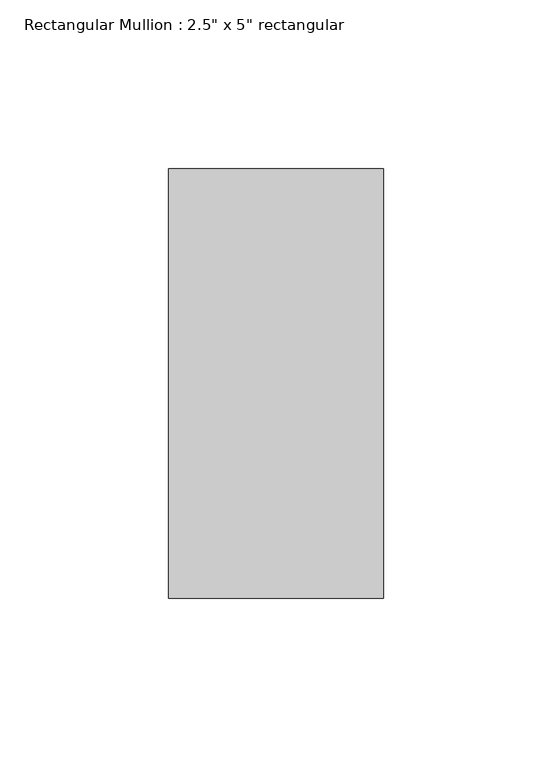
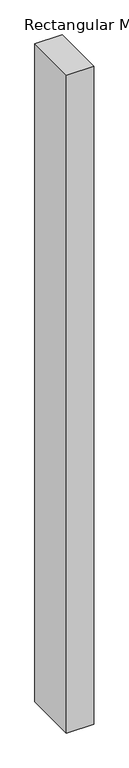
"""IFC4 building model written with IfcOpenShell, lengths in millimetres: member geometry."""

from ifc_helpers import new_model, si_unit, frame, origin, place, context, project, spatial, polyline, outline, extrude, source, transform, mapped, element, save


def member_7862cfa9(model_context):
    return source(origin(), model_context, "Body", "SweptSolid", [
        extrude(outline(polyline([(0.0, 63.5), (0.0, -63.5), (-63.5, -63.5), (-63.5, 63.5), (0.0, 63.5)])), frame((0.0, 0.0, -1618.023499), z_axis=(0.0, 0.0, 1.0), x_axis=(1.0, 0.0, 0.0)), (0.0, 0.0, 1.0), 1618.023499),
    ])


if __name__ == "__main__":
    model = new_model("IFC4")
    model_context = context("Model", 3, world=origin())
    ifc_project = project(units=[si_unit("LENGTHUNIT", "METRE", prefix="MILLI")], contexts=[model_context])
    site = spatial("IfcSite", under=ifc_project)
    building = spatial("IfcBuilding", under=site)
    placement = place(None, origin())
    member_shape = member_7862cfa9(model_context)
    element("IfcMember", 1, ObjectType="Rectangular Mullion : 2.5\" x 5\" rectangular", at=placement, inside=building, context=model_context, shape_type="MappedRepresentation", body=[
        mapped(member_shape, transform((0.0, 0.0, 0.0), x_axis=(1.0, 0.0, 0.0), y_axis=(0.0, 1.0, 0.0), z_axis=(0.0, 0.0, 1.0))),
    ])
    save(model, "model.ifc")

# Revit data of these elements
# Type "Rectangular Mullion : 2.5\" x 5\" rectangular"
#   built-in parameter 1007304 = 0.416667 (stored number, unit not read)
#   built-in parameter 1007301 = 0.104167 (stored number, unit not read)
#   built-in parameter 1007300 = 0.104167 (stored number, unit not read)
# Element 1 (IfcMember, "Rectangular Mullion : 2.5\" x 5\" rectangular")
#   Materials on its faces: "Aluminum"
# Materials
#   "Aluminum": class "Metal", colour RGB 247 247 247, transparency 0, Description = "Aluminum 6061", Cost = 0
